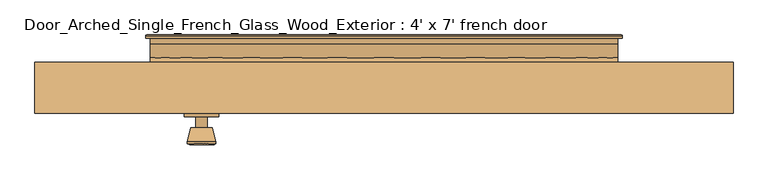
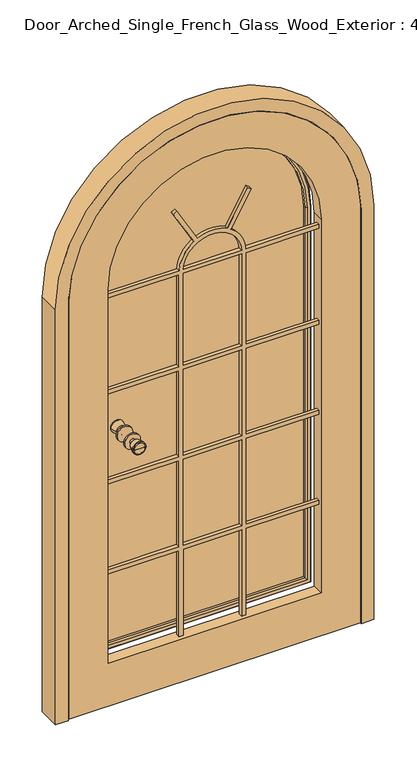
"""IFC4 building model written with IfcOpenShell, lengths in millimetres: door geometry, Door_Arched_Single_French_Glass_Wood_Exterior : 4' x 7' french door."""

from ifc_helpers import new_model, si_unit, point, frame, frame_2d, origin, place, context, project, spatial, polyline, circle_curve, ellipse_curve, trimmed, segment, composite_curve, outline, extrude, source, transform, mapped, element, save
from ifc_brep_helpers import plane_surface, cylinder_surface, revolved_surface, advanced_brep


def door_arched_single_french_glass_wood_exterior_4_x_7_french_5c4dec95(model_context):
    return source(origin(), model_context, "Body", "SolidModel", [
        advanced_brep(
        [(-318.5, -56.5, 1050.0), (-308.5, -56.5, 1050.0), (-328.5, -56.5, 1050.0), (-298.0241324, -105.5, 1050.0), (-318.5, -105.5, 1050.0), (-338.9758676, -105.5, 1050.0), (-293.5, -103.6721319, 1050.0), (-343.5, -103.6721319, 1050.0), (-293.5, -100.2084537, 1050.0), (-343.5, -100.2084537, 1050.0), (-299.863764, -75.5, 1050.0), (-337.136236, -75.5, 1050.0), (-308.5, -75.5, 1050.0), (-328.5, -75.5, 1050.0)],
        [
            (0, 1),
            (1, 2, circle_curve(frame((-318.5, -56.5, 1050.0), z_axis=(0.0, 1.0, 0.0), x_axis=(-1.0, 0.0, 0.0)), 10.0)),
            (2, 0),
            (2, 1, circle_curve(frame((-318.5, -56.5, 1050.0), z_axis=(0.0, 1.0, 0.0), x_axis=(-1.0, 0.0, 0.0)), 10.0)),
            (3, 4),
            (4, 5),
            (5, 3, circle_curve(frame((-318.5, -105.5, 1050.0), z_axis=(0.0, -1.0, 0.0), x_axis=(-1.0, 0.0, 0.0)), 20.4758676)),
            (3, 5, circle_curve(frame((-318.5, -105.5, 1050.0), z_axis=(0.0, -1.0, 0.0), x_axis=(-1.0, 0.0, 0.0)), 20.4758676)),
            (6, 3),
            (5, 7),
            (7, 6, circle_curve(frame((-318.5, -103.6721319, 1050.0), z_axis=(0.0, -1.0, 0.0), x_axis=(-1.0, 0.0, 0.0)), 25.0)),
            (6, 7, circle_curve(frame((-318.5, -103.6721319, 1050.0), z_axis=(0.0, -1.0, 0.0), x_axis=(-1.0, 0.0, 0.0)), 25.0)),
            (8, 6),
            (7, 9),
            (9, 8, circle_curve(frame((-318.5, -100.2084537, 1050.0), z_axis=(0.0, -1.0, 0.0), x_axis=(-1.0, 0.0, 0.0)), 25.0)),
            (8, 9, circle_curve(frame((-318.5, -100.2084537, 1050.0), z_axis=(0.0, -1.0, 0.0), x_axis=(-1.0, 0.0, 0.0)), 25.0)),
            (10, 8),
            (9, 11),
            (11, 10, circle_curve(frame((-318.5, -75.5, 1050.0), z_axis=(0.0, -1.0, 0.0), x_axis=(-1.0, 0.0, 0.0)), 18.636236)),
            (10, 11, circle_curve(frame((-318.5, -75.5, 1050.0), z_axis=(0.0, -1.0, 0.0), x_axis=(-1.0, 0.0, 0.0)), 18.636236)),
            (12, 10),
            (11, 13),
            (13, 12, circle_curve(frame((-318.5, -75.5, 1050.0), z_axis=(0.0, -1.0, 0.0), x_axis=(-1.0, 0.0, 0.0)), 10.0)),
            (12, 13, circle_curve(frame((-318.5, -75.5, 1050.0), z_axis=(0.0, -1.0, 0.0), x_axis=(-1.0, 0.0, 0.0)), 10.0)),
            (1, 12),
            (13, 2),
        ],
        [
            plane_surface(frame((-318.5, -56.5, 1050.0), z_axis=(0.0, 1.0, 0.0), x_axis=(-1.0, 0.0, 0.0))),
            plane_surface(frame((-318.5, -105.5, 1050.0), z_axis=(0.0, -1.0, 0.0), x_axis=(-1.0, 0.0, 0.0))),
            revolved_surface(polyline([(-338.9758676, -105.5, 1050.0), (-343.5, -103.6721319, 1050.0)]), (-318.5, -56.5, 1050.0), (0.0, 1.0, 0.0)),
            cylinder_surface(frame((-318.5, -56.5, 1050.0), z_axis=(0.0, 1.0, 0.0), x_axis=(-1.0, 0.0, 0.0)), 25.0),
            revolved_surface(polyline([(-343.5, -100.2084537, 1050.0), (-337.136236, -75.5, 1050.0)]), (-318.5, -56.5, 1050.0), (0.0, 1.0, 0.0)),
            plane_surface(frame((-318.5, -75.5, 1050.0), z_axis=(0.0, 1.0, 0.0), x_axis=(-1.0, 0.0, 0.0))),
            cylinder_surface(frame((-318.5, -56.5, 1050.0), z_axis=(0.0, 1.0, 0.0), x_axis=(-1.0, 0.0, 0.0)), 10.0),
        ],
        [
            (0, [[1, 2, 3]]),
            (0, [[-3, 4, -1]]),
            (1, [[5, 6, 7]]),
            (1, [[-6, -5, 8]]),
            (2, [[9, -7, 10, 11]]),
            (2, [[-10, -8, -9, 12]]),
            (3, [[13, -11, 14, 15]]),
            (3, [[-14, -12, -13, 16]]),
            (4, [[17, -15, 18, 19]]),
            (4, [[-18, -16, -17, 20]]),
            (5, [[21, -19, 22, 23]]),
            (5, [[-22, -20, -21, 24]]),
            (6, [[25, -23, 26, -2]]),
            (6, [[-26, -24, -25, -4]]),
        ],
    ),
        extrude(outline(composite_curve([segment(trimmed(circle_curve(frame_2d((1050.0, -318.5)), 30.0), [point((1050.0, -348.5))], [point((1050.0, -288.5))], False, "CARTESIAN"), True, "CONTINUOUS"), segment(trimmed(circle_curve(frame_2d((1050.0, -318.5)), 30.0), [point((1050.0, -288.5))], [point((1050.0, -348.5))], False, "CARTESIAN"), True, "CONTINUOUS")], self_intersect=False)), frame((0.0, -56.5, 0.0), z_axis=(0.0, 1.0, 0.0), x_axis=(0.0, 0.0, 1.0)), (0.0, 0.0, 1.0), 6.0),
        advanced_brep(
        [(-318.5, -0.5, 1050.0), (-328.5, -0.5, 1050.0), (-308.5, -0.5, 1050.0), (-298.0241324, 48.5, 1050.0), (-338.9758676, 48.5, 1050.0), (-318.5, 48.5, 1050.0), (-293.5, 46.6721319, 1050.0), (-343.5, 46.6721319, 1050.0), (-293.5, 43.2084537, 1050.0), (-343.5, 43.2084537, 1050.0), (-299.863764, 18.5, 1050.0), (-337.136236, 18.5, 1050.0), (-308.5, 18.5, 1050.0), (-328.5, 18.5, 1050.0)],
        [
            (0, 1),
            (1, 2, circle_curve(frame((-318.5, -0.5, 1050.0), z_axis=(0.0, -1.0, 0.0), x_axis=(-1.0, 0.0, 0.0)), 10.0)),
            (2, 0),
            (2, 1, circle_curve(frame((-318.5, -0.5, 1050.0), z_axis=(0.0, -1.0, 0.0), x_axis=(-1.0, 0.0, 0.0)), 10.0)),
            (3, 4, circle_curve(frame((-318.5, 48.5, 1050.0), z_axis=(0.0, 1.0, 0.0), x_axis=(-1.0, 0.0, 0.0)), 20.4758676)),
            (4, 5),
            (5, 3),
            (4, 3, circle_curve(frame((-318.5, 48.5, 1050.0), z_axis=(0.0, 1.0, 0.0), x_axis=(-1.0, 0.0, 0.0)), 20.4758676)),
            (6, 7, circle_curve(frame((-318.5, 46.6721319, 1050.0), z_axis=(0.0, 1.0, 0.0), x_axis=(-1.0, 0.0, 0.0)), 25.0)),
            (7, 4),
            (3, 6),
            (7, 6, circle_curve(frame((-318.5, 46.6721319, 1050.0), z_axis=(0.0, 1.0, 0.0), x_axis=(-1.0, 0.0, 0.0)), 25.0)),
            (8, 9, circle_curve(frame((-318.5, 43.2084537, 1050.0), z_axis=(0.0, 1.0, 0.0), x_axis=(-1.0, 0.0, 0.0)), 25.0)),
            (9, 7),
            (6, 8),
            (9, 8, circle_curve(frame((-318.5, 43.2084537, 1050.0), z_axis=(0.0, 1.0, 0.0), x_axis=(-1.0, 0.0, 0.0)), 25.0)),
            (10, 11, circle_curve(frame((-318.5, 18.5, 1050.0), z_axis=(0.0, 1.0, 0.0), x_axis=(-1.0, 0.0, 0.0)), 18.636236)),
            (11, 9),
            (8, 10),
            (11, 10, circle_curve(frame((-318.5, 18.5, 1050.0), z_axis=(0.0, 1.0, 0.0), x_axis=(-1.0, 0.0, 0.0)), 18.636236)),
            (12, 13, circle_curve(frame((-318.5, 18.5, 1050.0), z_axis=(0.0, 1.0, 0.0), x_axis=(-1.0, 0.0, 0.0)), 10.0)),
            (13, 11),
            (10, 12),
            (13, 12, circle_curve(frame((-318.5, 18.5, 1050.0), z_axis=(0.0, 1.0, 0.0), x_axis=(-1.0, 0.0, 0.0)), 10.0)),
            (1, 13),
            (12, 2),
        ],
        [
            plane_surface(frame((-318.5, -0.5, 1050.0), z_axis=(0.0, -1.0, 0.0), x_axis=(-1.0, 0.0, 0.0))),
            plane_surface(frame((-318.5, 48.5, 1050.0), z_axis=(0.0, 1.0, 0.0), x_axis=(-1.0, 0.0, 0.0))),
            revolved_surface(polyline([(-338.9758676, 48.5, 1050.0), (-343.5, 46.6721319, 1050.0)]), (-318.5, -0.5, 1050.0), (0.0, -1.0, 0.0)),
            cylinder_surface(frame((-318.5, -0.5, 1050.0), z_axis=(0.0, -1.0, 0.0), x_axis=(-1.0, 0.0, 0.0)), 25.0),
            revolved_surface(polyline([(-343.5, 43.2084537, 1050.0), (-337.136236, 18.5, 1050.0)]), (-318.5, -0.5, 1050.0), (0.0, -1.0, 0.0)),
            plane_surface(frame((-318.5, 18.5, 1050.0), z_axis=(0.0, -1.0, 0.0), x_axis=(-1.0, 0.0, 0.0))),
            cylinder_surface(frame((-318.5, -0.5, 1050.0), z_axis=(0.0, -1.0, 0.0), x_axis=(-1.0, 0.0, 0.0)), 10.0),
        ],
        [
            (0, [[1, 2, 3]]),
            (0, [[-3, 4, -1]]),
            (1, [[5, 6, 7]]),
            (1, [[8, -7, -6]]),
            (2, [[9, 10, -5, 11]]),
            (2, [[12, -11, -8, -10]]),
            (3, [[13, 14, -9, 15]]),
            (3, [[16, -15, -12, -14]]),
            (4, [[17, 18, -13, 19]]),
            (4, [[20, -19, -16, -18]]),
            (5, [[21, 22, -17, 23]]),
            (5, [[24, -23, -20, -22]]),
            (6, [[-2, 25, -21, 26]]),
            (6, [[-4, -26, -24, -25]]),
        ],
    ),
        extrude(outline(composite_curve([segment(trimmed(circle_curve(frame_2d((1050.0, -318.5)), 30.0), [point((1050.0, -348.5))], [point((1050.0, -288.5))], False, "CARTESIAN"), True, "CONTINUOUS"), segment(trimmed(circle_curve(frame_2d((1050.0, -318.5)), 30.0), [point((1050.0, -288.5))], [point((1050.0, -348.5))], False, "CARTESIAN"), True, "CONTINUOUS")], self_intersect=False)), frame((0.0, -6.5, 0.0), z_axis=(0.0, 1.0, 0.0), x_axis=(0.0, 0.0, 1.0)), (0.0, 0.0, 1.0), 6.0),
        advanced_brep(
        [(539.1, 38.5, 0.0), (609.6, 38.5, 0.0), (609.6, -50.5, 0.0), (561.1, -50.5, 0.0), (561.1, -3.5, 0.0), (539.1, -3.5, 0.0), (539.1, 38.5, 1678.6), (-539.1, 38.5, 1678.6), (-539.1, 38.5, 0.0), (-609.6, 38.5, 0.0), (-609.6, 38.5, 1678.6), (609.6, 38.5, 1678.6), (609.6, -50.5, 1678.6), (-609.6, -50.5, 1678.6), (-609.6, -50.5, 0.0), (-561.1, -50.5, 0.0), (-561.1, -50.5, 1678.6), (561.1, -50.5, 1678.6), (561.1, -3.5, 1678.6), (-561.1, -3.5, 1678.6), (-561.1, -3.5, 0.0), (-539.1, -3.5, 0.0), (-539.1, -3.5, 1678.6), (539.1, -3.5, 1678.6)],
        [
            (0, 1),
            (1, 2),
            (2, 3),
            (3, 4),
            (4, 5),
            (5, 0),
            (0, 6),
            (6, 7, circle_curve(frame((0.0, 38.5, 1678.6), z_axis=(0.0, -1.0, 0.0), x_axis=(1.0, 0.0, 0.0)), 539.1)),
            (7, 8),
            (8, 9),
            (9, 10),
            (10, 11, circle_curve(frame((0.0, 38.5, 1678.6), z_axis=(0.0, 1.0, 0.0), x_axis=(1.0, 0.0, 0.0)), 609.6)),
            (11, 1),
            (11, 12),
            (12, 2),
            (12, 13, circle_curve(frame((0.0, -50.5, 1678.6), z_axis=(0.0, -1.0, 0.0), x_axis=(1.0, 0.0, 0.0)), 609.6)),
            (13, 14),
            (14, 15),
            (15, 16),
            (16, 17, circle_curve(frame((0.0, -50.5, 1678.6), z_axis=(0.0, 1.0, 0.0), x_axis=(1.0, 0.0, 0.0)), 561.1)),
            (17, 3),
            (17, 18),
            (18, 4),
            (18, 19, circle_curve(frame((0.0, -3.5, 1678.6), z_axis=(0.0, -1.0, 0.0), x_axis=(1.0, 0.0, 0.0)), 561.1)),
            (19, 20),
            (20, 21),
            (21, 22),
            (22, 23, circle_curve(frame((0.0, -3.5, 1678.6), z_axis=(0.0, 1.0, 0.0), x_axis=(1.0, 0.0, 0.0)), 539.1)),
            (23, 5),
            (23, 6),
            (7, 22),
            (21, 8),
            (20, 15),
            (14, 9),
            (13, 10),
            (19, 16),
        ],
        [
            plane_surface(frame((603.1, -59.9123976, 0.0), z_axis=(0.0, 0.0, -1.0), x_axis=(1.0, 0.0, 0.0))),
            plane_surface(frame((539.1, 38.5, 0.0), z_axis=(0.0, 1.0, 0.0), x_axis=(0.0, 0.0, 1.0))),
            plane_surface(frame((609.6, 38.5, 0.0), z_axis=(1.0, 0.0, 0.0), x_axis=(0.0, 0.0, 1.0))),
            plane_surface(frame((609.6, -50.5, 0.0), z_axis=(0.0, -1.0, 0.0), x_axis=(0.0, 0.0, 1.0))),
            plane_surface(frame((561.1, -50.5, 0.0), z_axis=(-1.0, 0.0, 0.0), x_axis=(0.0, 0.0, 1.0))),
            plane_surface(frame((561.1, -3.5, 0.0), z_axis=(0.0, -1.0, 0.0), x_axis=(0.0, 0.0, 1.0))),
            plane_surface(frame((539.1, -3.5, 0.0), z_axis=(-1.0, 0.0, 0.0), x_axis=(0.0, 0.0, 1.0))),
            plane_surface(frame((-539.1, -3.5, 1678.6), z_axis=(1.0, 0.0, 0.0), x_axis=(0.0, 0.0, -1.0))),
            plane_surface(frame((-603.1, -59.9123976, 0.0), z_axis=(0.0, 0.0, -1.0), x_axis=(-1.0, 0.0, 0.0))),
            plane_surface(frame((-609.6, 38.5, 1678.6), z_axis=(-1.0, 0.0, 0.0), x_axis=(0.0, 0.0, -1.0))),
            plane_surface(frame((-561.1, -50.5, 1678.6), z_axis=(1.0, 0.0, 0.0), x_axis=(0.0, 0.0, -1.0))),
            cylinder_surface(frame((0.0, 38.5, 1678.6), z_axis=(0.0, -1.0, 0.0), x_axis=(1.0, 0.0, 0.0)), 609.6),
            revolved_surface(polyline([(561.1, -50.5, 1678.6), (561.1, -3.5, 1678.6)]), (0.0, 38.5, 1678.6), (0.0, -1.0, 0.0)),
            revolved_surface(polyline([(539.1, -3.5, 1678.6), (539.1, 38.5, 1678.6)]), (0.0, 38.5, 1678.6), (0.0, -1.0, 0.0)),
        ],
        [
            (0, [[1, 2, 3, 4, 5, 6]]),
            (1, [[-1, 7, 8, 9, 10, 11, 12, 13]]),
            (2, [[-2, -13, 14, 15]]),
            (3, [[-3, -15, 16, 17, 18, 19, 20, 21]]),
            (4, [[-4, -21, 22, 23]]),
            (5, [[-5, -23, 24, 25, 26, 27, 28, 29]]),
            (6, [[-6, -29, 30, -7]]),
            (7, [[31, -27, 32, -9]]),
            (8, [[-32, -26, 33, -18, 34, -10]]),
            (9, [[35, -11, -34, -17]]),
            (10, [[36, -19, -33, -25]]),
            (11, [[-16, -14, -12, -35]]),
            (12, [[-24, -22, -20, -36]]),
            (13, [[-8, -30, -28, -31]]),
        ],
    ),
        extrude(outline(composite_curve([segment(trimmed(circle_curve(frame_2d((1692.1, 0.0)), 253.5), [point((1896.740356, 149.6147543))], [point((1905.7961472, 136.3679092))], False, "CARTESIAN"), True, "CONTINUOUS"), segment(polyline([(1905.7961472, 136.3679092), (1768.2345335, 56.9466745)]), True, "CONTINUOUS"), segment(trimmed(circle_curve(frame_2d((1653.6, 0.0)), 128.0), [point((1768.2345335, 56.9466745))], [point((1768.2345335, -56.9466745))], False, "CARTESIAN"), True, "CONTINUOUS"), segment(polyline([(1768.2345335, -56.9466745), (1905.7961472, -136.3679092)]), True, "CONTINUOUS"), segment(trimmed(circle_curve(frame_2d((1692.1, 0.0)), 253.5), [point((1905.7961472, -136.3679092))], [point((1896.740356, -149.6147543))], False, "CARTESIAN"), True, "CONTINUOUS"), segment(polyline([(1896.740356, -149.6147543), (1760.2345335, -70.8030809)]), True, "CONTINUOUS"), segment(trimmed(circle_curve(frame_2d((1653.6, 0.0)), 128.0), [point((1760.2345335, -70.8030809))], [point((1661.6, -127.7497554))], False, "CARTESIAN"), True, "CONTINUOUS"), segment(polyline([(1661.6, -127.7497554), (1661.6, -408.1), (1645.6, -408.1), (1645.6, -128.0), (1273.5, -128.0), (1273.5, -408.1), (1257.5, -408.1), (1257.5, -128.0), (909.0, -128.0), (909.0, -408.1), (893.0, -408.1), (893.0, -128.0), (544.5, -128.0), (544.5, -408.1), (528.5, -408.1), (528.5, -128.0), (179.0, -128.0), (179.0, -112.0), (528.5, -112.0), (528.5, 112.0), (179.0, 112.0), (179.0, 128.0), (528.5, 128.0), (528.5, 408.1), (544.5, 408.1), (544.5, 128.0), (893.0, 128.0), (893.0, 408.1), (909.0, 408.1), (909.0, 128.0), (1257.5, 128.0), (1257.5, 408.1), (1273.5, 408.1), (1273.5, 128.0), (1645.6, 128.0), (1645.6, 408.1), (1661.6, 408.1), (1661.6, 127.7497554)]), True, "CONTINUOUS"), segment(trimmed(circle_curve(frame_2d((1653.6, 0.0)), 128.0), [point((1661.6, 127.7497554))], [point((1760.2345335, 70.8030809))], False, "CARTESIAN"), True, "CONTINUOUS"), segment(polyline([(1760.2345335, 70.8030809), (1896.740356, 149.6147543)]), True, "CONTINUOUS")], self_intersect=False), holes=[polyline([(893.0, -112.0), (893.0, 112.0), (544.5, 112.0), (544.5, -112.0), (893.0, -112.0)]), polyline([(1257.5, 112.0), (909.0, 112.0), (909.0, -112.0), (1257.5, -112.0), (1257.5, 112.0)]), composite_curve([segment(trimmed(circle_curve(frame_2d((1653.6, 0.0)), 112.0), [point((1661.6, -111.7139204))], [point((1661.6, 111.7139204))], True, "CARTESIAN"), True, "CONTINUOUS"), segment(polyline([(1661.6, 111.7139204), (1661.6, -111.7139204)]), True, "CONTINUOUS")], self_intersect=False), polyline([(1645.6, -112.0), (1645.6, 112.0), (1273.5, 112.0), (1273.5, -112.0), (1645.6, -112.0)])]), frame((0.0, -35.6484532, 0.0), z_axis=(0.0, 1.0, 0.0), x_axis=(0.0, 0.0, 1.0)), (0.0, 0.0, 1.0), 14.5359085),
        extrude(outline(composite_curve([segment(polyline([(4.0, 558.1), (1727.8950302, 558.1)]), True, "CONTINUOUS"), segment(trimmed(circle_curve(frame_2d((1678.6, 0.0)), 560.2727996), [point((1727.8950302, 558.1))], [point((1715.9714663, -559.0250294))], False, "CARTESIAN"), True, "CONTINUOUS"), segment(polyline([(1715.9714663, -559.0250294), (4.0, -559.0250294), (4.0, 558.1)]), True, "CONTINUOUS")], self_intersect=False), holes=[composite_curve([segment(polyline([(179.0, -408.1), (1692.1, -408.1)]), True, "CONTINUOUS"), segment(trimmed(circle_curve(frame_2d((1692.1, 0.0)), 408.1), [point((1692.1, -408.1))], [point((1692.1, 408.1))], True, "CARTESIAN"), True, "CONTINUOUS"), segment(polyline([(1692.1, 408.1), (179.0, 408.1), (179.0, -408.1)]), True, "CONTINUOUS")], self_intersect=False)]), frame((0.0, -50.5, 0.0), z_axis=(0.0, 1.0, 0.0), x_axis=(0.0, 0.0, 1.0)), (0.0, 0.0, 1.0), 44.0),
        extrude(outline(composite_curve([segment(polyline([(179.0, -408.1), (179.0, 408.1), (1692.1, 408.1)]), True, "CONTINUOUS"), segment(trimmed(circle_curve(frame_2d((1692.1, 0.0)), 408.1), [point((1692.1, 408.1))], [point((1692.1, -408.1))], False, "CARTESIAN"), True, "CONTINUOUS"), segment(polyline([(1692.1, -408.1), (179.0, -408.1)]), True, "CONTINUOUS")], self_intersect=False)), frame((0.0, 46.0, 0.0), z_axis=(0.0, 1.0, 0.0), x_axis=(0.0, 0.0, 1.0)), (0.0, 0.0, 1.0), 24.0),
        advanced_brep(
        [(-416.1, 84.0, 171.0), (-416.1, 80.0, 171.0), (-416.1, 80.0, 1692.1), (-416.1, 84.0, 1692.1), (-414.1, 86.0, 173.0), (-414.1, 86.0, 1692.1), (-396.1, 81.0, 191.0), (-401.1, 86.0, 186.0), (-401.1, 86.0, 1692.1), (-396.1, 81.0, 1692.1), (-396.1, 70.0, 191.0), (-396.1, 70.0, 1692.1), (-408.1, 80.0, 179.0), (-408.1, 70.0, 179.0), (-408.1, 70.0, 1692.1), (-408.1, 80.0, 1692.1), (416.1, 84.0, 1692.1), (416.1, 80.0, 1692.1), (414.1, 86.0, 1692.1), (414.1, 86.0, 173.0), (401.1, 86.0, 1692.1), (401.1, 86.0, 186.0), (396.1, 81.0, 1692.1), (396.1, 70.0, 1692.1), (408.1, 70.0, 1692.1), (408.1, 70.0, 179.0), (396.1, 70.0, 191.0), (408.1, 80.0, 1692.1), (416.1, 80.0, 171.0), (408.1, 80.0, 179.0), (416.1, 84.0, 171.0), (396.1, 81.0, 191.0)],
        [
            (0, 1),
            (1, 2),
            (2, 3),
            (3, 0),
            (4, 0, ellipse_curve(frame((-414.1, 84.0, 173.0), z_axis=(-0.7071067811865475, 0.0, 0.7071067811865475), x_axis=(-0.7071067811865474, 0.0, -0.7071067811865476)), 2.8284271, 2.0)),
            (3, 5, circle_curve(frame((-414.1, 84.0, 1692.1), z_axis=(0.0, 0.0, -1.0), x_axis=(-1.0, 0.0, 0.0)), 2.0)),
            (5, 4),
            (6, 7, ellipse_curve(frame((-401.1, 81.0, 186.0), z_axis=(-0.7071067811865475, 0.0, 0.7071067811865475), x_axis=(-0.7071067811865474, 0.0, -0.7071067811865476)), 7.0710678, 5.0)),
            (7, 8),
            (8, 9, circle_curve(frame((-401.1, 81.0, 1692.1), z_axis=(0.0, 0.0, -1.0), x_axis=(-1.0, 0.0, 0.0)), 5.0)),
            (9, 6),
            (10, 6),
            (9, 11),
            (11, 10),
            (12, 13),
            (13, 14),
            (14, 15),
            (15, 12),
            (16, 3, circle_curve(frame((0.0, 84.0, 1692.1), z_axis=(0.0, -1.0, 0.0), x_axis=(-1.0, 0.0, 0.0)), 416.1)),
            (2, 17, circle_curve(frame((0.0, 80.0, 1692.1), z_axis=(0.0, 1.0, 0.0), x_axis=(-1.0, 0.0, 0.0)), 416.1)),
            (17, 16),
            (18, 5, circle_curve(frame((0.0, 86.0, 1692.1), z_axis=(0.0, -1.0, 0.0), x_axis=(-1.0, 0.0, 0.0)), 414.1)),
            (16, 18, circle_curve(frame((414.1, 84.0, 1692.1), z_axis=(0.0, 0.0, 1.0), x_axis=(1.0, 0.0, 0.0)), 2.0)),
            (18, 19),
            (19, 4),
            (20, 8, circle_curve(frame((0.0, 86.0, 1692.1), z_axis=(0.0, -1.0, 0.0), x_axis=(-1.0, 0.0, 0.0)), 401.1)),
            (7, 21),
            (21, 20),
            (22, 9, circle_curve(frame((0.0, 81.0, 1692.1), z_axis=(0.0, -1.0, 0.0), x_axis=(-1.0, 0.0, 0.0)), 396.1)),
            (20, 22, circle_curve(frame((401.1, 81.0, 1692.1), z_axis=(0.0, 0.0, 1.0), x_axis=(1.0, 0.0, 0.0)), 5.0)),
            (23, 11, circle_curve(frame((0.0, 70.0, 1692.1), z_axis=(0.0, -1.0, 0.0), x_axis=(-1.0, 0.0, 0.0)), 396.1)),
            (22, 23),
            (24, 14, circle_curve(frame((0.0, 70.0, 1692.1), z_axis=(0.0, -1.0, 0.0), x_axis=(-1.0, 0.0, 0.0)), 408.1)),
            (13, 25),
            (25, 24),
            (23, 26),
            (26, 10),
            (27, 15, circle_curve(frame((0.0, 80.0, 1692.1), z_axis=(0.0, -1.0, 0.0), x_axis=(-1.0, 0.0, 0.0)), 408.1)),
            (24, 27),
            (1, 28),
            (28, 17),
            (27, 29),
            (29, 12),
            (28, 30),
            (30, 16),
            (30, 19, ellipse_curve(frame((414.1, 84.0, 173.0), z_axis=(0.7071067811865475, 0.0, 0.7071067811865475), x_axis=(-0.7071067811865474, 0.0, 0.7071067811865476)), 2.8284271, 2.0)),
            (21, 31, ellipse_curve(frame((401.1, 81.0, 186.0), z_axis=(0.7071067811865475, 0.0, 0.7071067811865475), x_axis=(-0.7071067811865474, 0.0, 0.7071067811865476)), 7.0710678, 5.0)),
            (31, 22),
            (31, 26),
            (25, 29),
            (0, 30),
            (6, 31),
        ],
        [
            plane_surface(frame((-416.1, 80.0, 171.0), z_axis=(-1.0, 0.0, 0.0), x_axis=(0.0, 0.0, 1.0))),
            cylinder_surface(frame((-414.1, 84.0, 179.0), z_axis=(0.0, 0.0, -1.0), x_axis=(-1.0, 0.0, 0.0)), 2.0),
            cylinder_surface(frame((-401.1, 81.0, 179.0), z_axis=(0.0, 0.0, -1.0), x_axis=(-1.0, 0.0, 0.0)), 5.0),
            plane_surface(frame((-396.1, 81.0, 191.0), z_axis=(1.0, 0.0, 0.0), x_axis=(0.0, 0.0, 1.0))),
            plane_surface(frame((-408.1, 70.0, 179.0), z_axis=(-1.0, 0.0, 0.0), x_axis=(0.0, 0.0, 1.0))),
            cylinder_surface(frame((0.0, 80.0, 1692.1), z_axis=(0.0, 1.0, 0.0), x_axis=(-1.0, 0.0, 0.0)), 416.1),
            revolved_surface(trimmed(ellipse_curve(frame((-414.1, 84.0, 1692.1), z_axis=(0.0, 0.0, -1.0), x_axis=(-1.0, 0.0, 0.0)), 2.0, 2.0), [point((-416.1, 84.0, 1692.1))], [point((-414.1, 86.0, 1692.1))], True, "CARTESIAN"), (0.0, 80.0, 1692.1), (0.0, 1.0, 0.0)),
            plane_surface(frame((0.0, 86.0, 1692.1), z_axis=(0.0, 1.0, 0.0), x_axis=(-1.0, 0.0, 0.0))),
            revolved_surface(trimmed(ellipse_curve(frame((-401.1, 81.0, 1692.1), z_axis=(0.0, 0.0, -1.0), x_axis=(-1.0, 0.0, 0.0)), 5.0, 5.0), [point((-401.1, 86.0, 1692.1))], [point((-396.1, 81.0, 1692.1))], True, "CARTESIAN"), (0.0, 80.0, 1692.1), (0.0, 1.0, 0.0)),
            revolved_surface(polyline([(-396.1, 81.0, 1692.1), (-396.1, 70.0, 1692.1)]), (0.0, 80.0, 1692.1), (0.0, 1.0, 0.0)),
            plane_surface(frame((0.0, 70.0, 1692.1), z_axis=(0.0, -1.0, 0.0), x_axis=(-1.0, 0.0, 0.0))),
            cylinder_surface(frame((0.0, 80.0, 1692.1), z_axis=(0.0, 1.0, 0.0), x_axis=(-1.0, 0.0, 0.0)), 408.1),
            plane_surface(frame((0.0, 80.0, 1692.1), z_axis=(0.0, -1.0, 0.0), x_axis=(-1.0, 0.0, 0.0))),
            plane_surface(frame((416.1, 80.0, 1692.1), z_axis=(1.0, 0.0, 0.0), x_axis=(0.0, 0.0, -1.0))),
            cylinder_surface(frame((414.1, 84.0, 1692.1), z_axis=(0.0, 0.0, 1.0), x_axis=(1.0, 0.0, 0.0)), 2.0),
            cylinder_surface(frame((401.1, 81.0, 1692.1), z_axis=(0.0, 0.0, 1.0), x_axis=(1.0, 0.0, 0.0)), 5.0),
            plane_surface(frame((396.1, 81.0, 1692.1), z_axis=(-1.0, 0.0, 0.0), x_axis=(0.0, 0.0, -1.0))),
            plane_surface(frame((408.1, 70.0, 1692.1), z_axis=(1.0, 0.0, 0.0), x_axis=(0.0, 0.0, -1.0))),
            plane_surface(frame((416.1, 80.0, 171.0), z_axis=(0.0, 0.0, -1.0), x_axis=(-1.0, 0.0, 0.0))),
            cylinder_surface(frame((408.1, 84.0, 173.0), z_axis=(1.0, 0.0, 0.0), x_axis=(0.0, 0.0, -1.0)), 2.0),
            cylinder_surface(frame((408.1, 81.0, 186.0), z_axis=(1.0, 0.0, 0.0), x_axis=(0.0, 0.0, -1.0)), 5.0),
            plane_surface(frame((396.1, 81.0, 191.0), z_axis=(0.0, 0.0, 1.0), x_axis=(-1.0, 0.0, 0.0))),
            plane_surface(frame((408.1, 70.0, 179.0), z_axis=(0.0, 0.0, -1.0), x_axis=(-1.0, 0.0, 0.0))),
        ],
        [
            (0, [[1, 2, 3, 4]]),
            (1, [[5, -4, 6, 7]]),
            (2, [[8, 9, 10, 11]]),
            (3, [[12, -11, 13, 14]]),
            (4, [[15, 16, 17, 18]]),
            (5, [[19, -3, 20, 21]]),
            (6, [[22, -6, -19, 23]]),
            (7, [[24, 25, -7, -22], [26, -9, 27, 28]]),
            (8, [[29, -10, -26, 30]]),
            (9, [[31, -13, -29, 32]]),
            (10, [[33, -16, 34, 35], [36, 37, -14, -31]]),
            (11, [[38, -17, -33, 39]]),
            (12, [[-20, -2, 40, 41], [42, 43, -18, -38]]),
            (13, [[-21, -41, 44, 45]]),
            (14, [[-23, -45, 46, -24]]),
            (15, [[-30, -28, 47, 48]]),
            (16, [[-32, -48, 49, -36]]),
            (17, [[-39, -35, 50, -42]]),
            (18, [[-44, -40, -1, 51]]),
            (19, [[-46, -51, -5, -25]]),
            (20, [[-47, -27, -8, 52]]),
            (21, [[-49, -52, -12, -37]]),
            (22, [[-50, -34, -15, -43]]),
        ],
    ),
        advanced_brep(
        [(416.1, 32.0, 171.0), (416.1, 36.0, 171.0), (416.1, 36.0, 1692.1), (416.1, 32.0, 1692.1), (414.1, 30.0, 173.0), (414.1, 30.0, 1692.1), (396.1, 35.0, 191.0), (401.1, 30.0, 186.0), (401.1, 30.0, 1692.1), (396.1, 35.0, 1692.1), (396.1, 46.0, 191.0), (396.1, 46.0, 1692.1), (408.1, 36.0, 179.0), (408.1, 46.0, 179.0), (408.1, 46.0, 1692.1), (408.1, 36.0, 1692.1), (-416.1, 32.0, 1692.1), (-416.1, 36.0, 1692.1), (-414.1, 30.0, 1692.1), (-414.1, 30.0, 173.0), (-401.1, 30.0, 1692.1), (-401.1, 30.0, 186.0), (-396.1, 35.0, 1692.1), (-396.1, 46.0, 1692.1), (-408.1, 46.0, 1692.1), (-408.1, 46.0, 179.0), (-396.1, 46.0, 191.0), (-408.1, 36.0, 1692.1), (-416.1, 36.0, 171.0), (-408.1, 36.0, 179.0), (-416.1, 32.0, 171.0), (-396.1, 35.0, 191.0)],
        [
            (0, 1),
            (1, 2),
            (2, 3),
            (3, 0),
            (4, 0, ellipse_curve(frame((414.1, 32.0, 173.0), z_axis=(0.7071067811865475, 0.0, 0.7071067811865475), x_axis=(0.7071067811865474, 0.0, -0.7071067811865476)), 2.8284271, 2.0)),
            (3, 5, circle_curve(frame((414.1, 32.0, 1692.1), z_axis=(0.0, 0.0, -1.0), x_axis=(1.0, 0.0, 0.0)), 2.0)),
            (5, 4),
            (6, 7, ellipse_curve(frame((401.1, 35.0, 186.0), z_axis=(0.7071067811865475, 0.0, 0.7071067811865475), x_axis=(0.7071067811865474, 0.0, -0.7071067811865476)), 7.0710678, 5.0)),
            (7, 8),
            (8, 9, circle_curve(frame((401.1, 35.0, 1692.1), z_axis=(0.0, 0.0, -1.0), x_axis=(1.0, 0.0, 0.0)), 5.0)),
            (9, 6),
            (10, 6),
            (9, 11),
            (11, 10),
            (12, 13),
            (13, 14),
            (14, 15),
            (15, 12),
            (16, 3, circle_curve(frame((0.0, 32.0, 1692.1), z_axis=(0.0, 1.0, 0.0), x_axis=(1.0, 0.0, 0.0)), 416.1)),
            (2, 17, circle_curve(frame((0.0, 36.0, 1692.1), z_axis=(0.0, -1.0, 0.0), x_axis=(1.0, 0.0, 0.0)), 416.1)),
            (17, 16),
            (18, 5, circle_curve(frame((0.0, 30.0, 1692.1), z_axis=(0.0, 1.0, 0.0), x_axis=(1.0, 0.0, 0.0)), 414.1)),
            (16, 18, circle_curve(frame((-414.1, 32.0, 1692.1), z_axis=(0.0, 0.0, 1.0), x_axis=(-1.0, 0.0, 0.0)), 2.0)),
            (18, 19),
            (19, 4),
            (20, 8, circle_curve(frame((0.0, 30.0, 1692.1), z_axis=(0.0, 1.0, 0.0), x_axis=(1.0, 0.0, 0.0)), 401.1)),
            (7, 21),
            (21, 20),
            (22, 9, circle_curve(frame((0.0, 35.0, 1692.1), z_axis=(0.0, 1.0, 0.0), x_axis=(1.0, 0.0, 0.0)), 396.1)),
            (20, 22, circle_curve(frame((-401.1, 35.0, 1692.1), z_axis=(0.0, 0.0, 1.0), x_axis=(-1.0, 0.0, 0.0)), 5.0)),
            (23, 11, circle_curve(frame((0.0, 46.0, 1692.1), z_axis=(0.0, 1.0, 0.0), x_axis=(1.0, 0.0, 0.0)), 396.1)),
            (22, 23),
            (24, 14, circle_curve(frame((0.0, 46.0, 1692.1), z_axis=(0.0, 1.0, 0.0), x_axis=(1.0, 0.0, 0.0)), 408.1)),
            (13, 25),
            (25, 24),
            (23, 26),
            (26, 10),
            (27, 15, circle_curve(frame((0.0, 36.0, 1692.1), z_axis=(0.0, 1.0, 0.0), x_axis=(1.0, 0.0, 0.0)), 408.1)),
            (24, 27),
            (1, 28),
            (28, 17),
            (27, 29),
            (29, 12),
            (28, 30),
            (30, 16),
            (30, 19, ellipse_curve(frame((-414.1, 32.0, 173.0), z_axis=(-0.7071067811865475, 0.0, 0.7071067811865475), x_axis=(0.7071067811865474, 0.0, 0.7071067811865476)), 2.8284271, 2.0)),
            (21, 31, ellipse_curve(frame((-401.1, 35.0, 186.0), z_axis=(-0.7071067811865475, 0.0, 0.7071067811865475), x_axis=(0.7071067811865474, 0.0, 0.7071067811865476)), 7.0710678, 5.0)),
            (31, 22),
            (31, 26),
            (25, 29),
            (0, 30),
            (6, 31),
        ],
        [
            plane_surface(frame((416.1, 36.0, 171.0), z_axis=(1.0, 0.0, 0.0), x_axis=(0.0, 0.0, 1.0))),
            cylinder_surface(frame((414.1, 32.0, 179.0), z_axis=(0.0, 0.0, -1.0), x_axis=(1.0, 0.0, 0.0)), 2.0),
            cylinder_surface(frame((401.1, 35.0, 179.0), z_axis=(0.0, 0.0, -1.0), x_axis=(1.0, 0.0, 0.0)), 5.0),
            plane_surface(frame((396.1, 35.0, 191.0), z_axis=(-1.0, 0.0, 0.0), x_axis=(0.0, 0.0, 1.0))),
            plane_surface(frame((408.1, 46.0, 179.0), z_axis=(1.0, 0.0, 0.0), x_axis=(0.0, 0.0, 1.0))),
            cylinder_surface(frame((0.0, 36.0, 1692.1), z_axis=(0.0, -1.0, 0.0), x_axis=(1.0, 0.0, 0.0)), 416.1),
            revolved_surface(trimmed(ellipse_curve(frame((414.1, 32.0, 1692.1), z_axis=(0.0, 0.0, -1.0), x_axis=(1.0, 0.0, 0.0)), 2.0, 2.0), [point((416.1, 32.0, 1692.1))], [point((414.1, 30.0, 1692.1))], True, "CARTESIAN"), (0.0, 36.0, 1692.1), (0.0, -1.0, 0.0)),
            plane_surface(frame((0.0, 30.0, 1692.1), z_axis=(0.0, -1.0, 0.0), x_axis=(1.0, 0.0, 0.0))),
            revolved_surface(trimmed(ellipse_curve(frame((401.1, 35.0, 1692.1), z_axis=(0.0, 0.0, -1.0), x_axis=(1.0, 0.0, 0.0)), 5.0, 5.0), [point((401.1, 30.0, 1692.1))], [point((396.1, 35.0, 1692.1))], True, "CARTESIAN"), (0.0, 36.0, 1692.1), (0.0, -1.0, 0.0)),
            revolved_surface(polyline([(396.1, 35.0, 1692.1), (396.1, 46.0, 1692.1)]), (0.0, 36.0, 1692.1), (0.0, -1.0, 0.0)),
            plane_surface(frame((0.0, 46.0, 1692.1), z_axis=(0.0, 1.0, 0.0), x_axis=(1.0, 0.0, 0.0))),
            cylinder_surface(frame((0.0, 36.0, 1692.1), z_axis=(0.0, -1.0, 0.0), x_axis=(1.0, 0.0, 0.0)), 408.1),
            plane_surface(frame((0.0, 36.0, 1692.1), z_axis=(0.0, 1.0, 0.0), x_axis=(1.0, 0.0, 0.0))),
            plane_surface(frame((-416.1, 36.0, 1692.1), z_axis=(-1.0, 0.0, 0.0), x_axis=(0.0, 0.0, -1.0))),
            cylinder_surface(frame((-414.1, 32.0, 1692.1), z_axis=(0.0, 0.0, 1.0), x_axis=(-1.0, 0.0, 0.0)), 2.0),
            cylinder_surface(frame((-401.1, 35.0, 1692.1), z_axis=(0.0, 0.0, 1.0), x_axis=(-1.0, 0.0, 0.0)), 5.0),
            plane_surface(frame((-396.1, 35.0, 1692.1), z_axis=(1.0, 0.0, 0.0), x_axis=(0.0, 0.0, -1.0))),
            plane_surface(frame((-408.1, 46.0, 1692.1), z_axis=(-1.0, 0.0, 0.0), x_axis=(0.0, 0.0, -1.0))),
            plane_surface(frame((-416.1, 36.0, 171.0), z_axis=(0.0, 0.0, -1.0), x_axis=(1.0, 0.0, 0.0))),
            cylinder_surface(frame((-408.1, 32.0, 173.0), z_axis=(-1.0, 0.0, 0.0), x_axis=(0.0, 0.0, -1.0)), 2.0),
            cylinder_surface(frame((-408.1, 35.0, 186.0), z_axis=(-1.0, 0.0, 0.0), x_axis=(0.0, 0.0, -1.0)), 5.0),
            plane_surface(frame((-396.1, 35.0, 191.0), z_axis=(0.0, 0.0, 1.0), x_axis=(1.0, 0.0, 0.0))),
            plane_surface(frame((-408.1, 46.0, 179.0), z_axis=(0.0, 0.0, -1.0), x_axis=(1.0, 0.0, 0.0))),
        ],
        [
            (0, [[1, 2, 3, 4]]),
            (1, [[5, -4, 6, 7]]),
            (2, [[8, 9, 10, 11]]),
            (3, [[12, -11, 13, 14]]),
            (4, [[15, 16, 17, 18]]),
            (5, [[19, -3, 20, 21]]),
            (6, [[22, -6, -19, 23]]),
            (7, [[24, 25, -7, -22], [26, -9, 27, 28]]),
            (8, [[29, -10, -26, 30]]),
            (9, [[31, -13, -29, 32]]),
            (10, [[33, -16, 34, 35], [36, 37, -14, -31]]),
            (11, [[38, -17, -33, 39]]),
            (12, [[-20, -2, 40, 41], [42, 43, -18, -38]]),
            (13, [[-21, -41, 44, 45]]),
            (14, [[-23, -45, 46, -24]]),
            (15, [[-30, -28, 47, 48]]),
            (16, [[-32, -48, 49, -36]]),
            (17, [[-39, -35, 50, -42]]),
            (18, [[-44, -40, -1, 51]]),
            (19, [[-46, -51, -5, -25]]),
            (20, [[-47, -27, -8, 52]]),
            (21, [[-49, -52, -12, -37]]),
            (22, [[-50, -34, -15, -43]]),
        ],
    ),
    ])


if __name__ == "__main__":
    model = new_model("IFC4")
    model_context = context("Model", 3, world=origin())
    ifc_project = project(units=[si_unit("LENGTHUNIT", "METRE", prefix="MILLI")], contexts=[model_context])
    site = spatial("IfcSite", under=ifc_project)
    building = spatial("IfcBuilding", under=site)
    placement = place(None, origin())
    door_arched_single_french_glass_wood_exterior_4_x_7_french_shape = door_arched_single_french_glass_wood_exterior_4_x_7_french_5c4dec95(model_context)
    element("IfcDoor", 1, ObjectType="Door_Arched_Single_French_Glass_Wood_Exterior : 4' x 7' french door", at=placement, inside=building, context=model_context, shape_type="MappedRepresentation", body=[
        mapped(door_arched_single_french_glass_wood_exterior_4_x_7_french_shape, transform((0.0, 0.0, 0.0), x_axis=(1.0, 0.0, 0.0), y_axis=(0.0, 1.0, 0.0), z_axis=(0.0, 0.0, 1.0))),
    ])
    save(model, "model.ifc")

# Revit data of these elements
# Type "Door_Arched_Single_French_Glass_Wood_Exterior : 4' x 7' french door"
#   Type Mark = "17"
#   Type Comments = "External Single"
#   Operation = "SingleSwingRight"
#   Keynote = "L20"
#   Analytic Construction = "<None>"
#   Wrap Layers (Int) from Ext = 0' - 6.98819"
#   Wrap Layers (Ext) from Ext = 0' - 4.03543"
#   Thickness = 0' - 1.73228"
#   Stile Shutting = 0' - 5.90551"
#   Stile - Top Rail = 0' - 5.90551"
#   Stile - Hanging = 0' - 5.90551"
#   Stile - Bottom Rail = 0' - 6.88976"
#   Rough Width = 4' - 0"
#   Rough Height = 7' - 0"
#   O/A Frame Width = 0' - 2.51969"
#   Handle Z Distance = 3' - 5.33858"
#   Glazing Thickness = 0' - 0.94488"
#   Glazing Bar Thickness = 0' - 0.7874"
#   FrameWidth = 0' - 1.65354"
#   FrameOffset - External = 0' - 0.98425"
#   FrameDepth = 0' - 3.50394"
#   Door Panel Width = 3' - 7.94488"
#   Handle X Distance = 0' - 2.95276"
#   Height = 7' - 0"
#   Structural Tolerance = 0' - 0.25591"
#   Tolerance = 0' - 0.11811"
#   Undercut = 0' - 0.15748"
#   Width = 4' - 0"
#   Door Panel Thickness = 0' - 1.73228"
#   Door Panel Height = 6' - 9.81496"
#   Cavity Closer Width = 0' - 1.9685"
#   Cavity Closer Offset from Ext = 0' - 4.03543"
#   Cavity Closer Depth = 0' - 3.34646"
#   Vis - Ironmongery = yes
#   Vis - Cavity Closers = yes
#   Define Thermal Properties by = 1
#   Material Glass = Door - Glazing
#   Handle Style = element 430241
#   Material Door = Door - Panel
#   Material Frame = BROWN
#   Material Ironmongery = Door - Handle
#   Function = (empty or 0)
#   Wall Closure = (empty or 0)
#   Assembly Code = ""
# Element 1 (IfcDoor, "Door_Arched_Single_French_Glass_Wood_Exterior : 4' x 7' french door")
#   Materials on its faces: "Door - Panel", "Door - Handle", "BROWN", "Door - Glazing"
# Materials
#   "Door - Glazing": colour RGB 218 227 224, transparency 0.85
#   "Door - Panel": class "Wood", colour RGB 210 159 95, transparency 0, Cost = 0
#   "BROWN": class "Generic", colour RGB 120 120 120, transparency 0, Cost = 0
#   "Door - Handle": colour RGB 0 0 0, transparency 0, Keynote = "P21"
